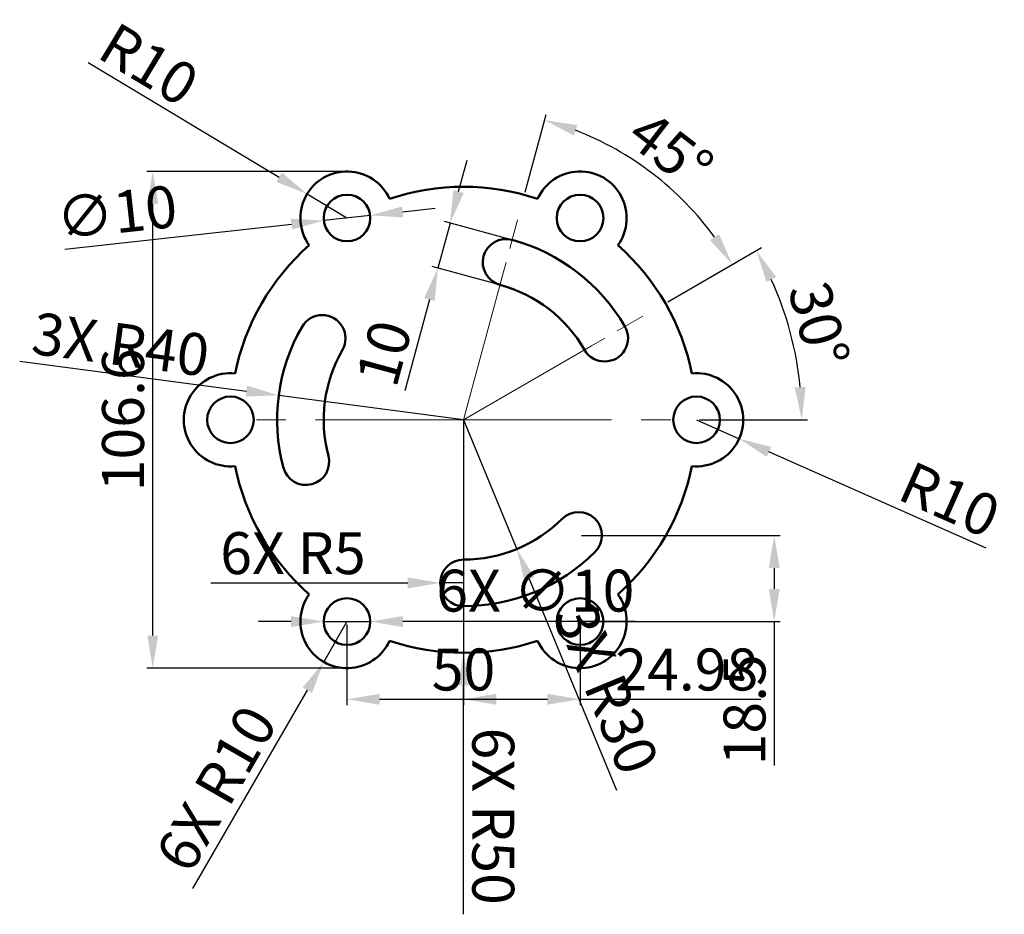
# Model space of a CAD drawing. Units: millimetres. Extents: x 2657 to 2869, y 1596 to 1788.
import ezdxf

# ---------------------------------------------------------------- set-up
doc = ezdxf.new("R2010")
doc.units = ezdxf.units.MM
doc.linetypes.add('CENTER', pattern=[50.8, 31.75, -6.35, 6.35, -6.35])
for name, color, linetype, lineweight in [('M-CNTR', 4, 'CENTER', 18), ('M-CONS', 8, 'Continuous', 13), ('M-DIMS', 2, 'Continuous', 25), ('M-OUTL', 7, 'Continuous', 50)]:
    doc.layers.add(name, color=color, linetype=linetype, lineweight=lineweight)
doc.styles.get("Standard").update_dxf_attribs({"font": 'arial.ttf'})
doc.dimstyles.new('ISO-25', dxfattribs={"dimtxt": 9, "dimasz": 7, "dimexe": 1.25, "dimexo": 0.625, "dimtad": 1, "dimtxsty": 'Standard', "dimcen": 2.5, "dimadec": 0, "dimazin": 0, "dimtfac": 1, "dimtmove": 0, "dimatfit": 3, "dimfxl": 1, "dimarcsym": 0})

# ---------------------------------------------------------------- blocks, each defined once
blk = doc.blocks.new('*D1')
at = {"layer": 'Defpoints', "color": 0, "transparency": 16777216}
for p in [(2765.66, 1750.34), (2799.73, 1749.16), (2795.9, 1727.1), (2752.61, 1702.07), (2752.61, 1702.07)]:
    blk.add_point(p, dxfattribs=at)
at = {"layer": 'M-DIMS', "color": 0, "lineweight": -2, "transparency": 16777216}
for p, q in [((2765.82, 1750.94), (2770.31, 1767.58)), ((2796.44, 1727.41), (2811.36, 1736.04))]:
    blk.add_line(p, q, dxfattribs=at)
blk.add_arc((2752.61, 1702.07), 66.61, 36.0596, 68.8542, dxfattribs=at)
at = {"layer": 'M-DIMS', "color": 0, "transparency": 16777216}
for points in [[(2776.28, 1763.09), (2777, 1765.3), (2769.99, 1766.37)], [(2807.44, 1741.91), (2805.48, 1740.64), (2810.28, 1735.41)]]:
    blk.add_solid(points, dxfattribs=at)
at = {"layer": 'M-DIMS', "color": 0, "transparency": 16777216, "insert": (2796.37, 1759.01), "char_height": 9, "attachment_point": 5, "rotation": 322.4569}
blk.add_mtext('45°', dxfattribs=at)
blk = doc.blocks.new('*D2')
at = {"layer": 'Defpoints', "color": 0, "transparency": 16777216}
for p in [(2795.9, 1727.1), (2824.08, 1714.69), (2752.61, 1702.07), (2752.61, 1702.07), (2802.61, 1702.07)]:
    blk.add_point(p, dxfattribs=at)
at = {"layer": 'M-DIMS', "color": 0, "lineweight": -2, "transparency": 16777216}
for p, q in [((2796.44, 1727.41), (2816.52, 1739.02)), ((2803.24, 1702.07), (2826.44, 1702.07))]:
    blk.add_line(p, q, dxfattribs=at)
blk.add_arc((2752.61, 1702.07), 72.58, 5.5283, 24.5074, dxfattribs=at)
at = {"layer": 'M-DIMS', "color": 0, "transparency": 16777216}
for points in [[(2817.61, 1731.64), (2819.69, 1732.71), (2815.44, 1738.4)], [(2826.02, 1709.12), (2823.69, 1709.01), (2825.19, 1702.07)]]:
    blk.add_solid(points, dxfattribs=at)
at = {"layer": 'M-DIMS', "color": 0, "transparency": 16777216, "insert": (2827.75, 1722.23), "char_height": 9, "attachment_point": 5, "rotation": 285.0179}
blk.add_mtext('30°', dxfattribs=at)
blk = doc.blocks.new('*D3')
at = {"layer": 'Defpoints', "color": 0, "transparency": 16777216}
for p in [(2763.05, 1740.68), (2747.12, 1734.63), (2760.44, 1731.03)]:
    blk.add_point(p, dxfattribs=at)
at = {"layer": 'M-DIMS', "color": 0, "lineweight": -2, "transparency": 16777216}
for p, q in [((2751.55, 1751.04), (2753.38, 1757.8)), ((2749.72, 1744.28), (2747.12, 1734.63)), ((2762.44, 1740.85), (2748.52, 1744.61)), ((2759.83, 1731.19), (2745.91, 1734.96)), ((2745.29, 1727.87), (2740, 1708.31))]:
    blk.add_line(p, q, dxfattribs=at)
at = {"layer": 'M-DIMS', "color": 0, "transparency": 16777216}
for points in [[(2750.42, 1751.35), (2752.68, 1750.74), (2749.72, 1744.28)], [(2744.16, 1728.18), (2746.42, 1727.57), (2747.12, 1734.63)]]:
    blk.add_solid(points, dxfattribs=at)
at = {"layer": 'M-DIMS', "color": 0, "transparency": 16777216, "insert": (2736.69, 1716.08), "char_height": 9, "attachment_point": 5, "rotation": 74.8781}
blk.add_mtext('10', dxfattribs=at)
blk = doc.blocks.new('*D4')
at = {"layer": 'Defpoints', "color": 0, "transparency": 16777216}
for p in [(2719.04, 1750.52), (2727.61, 1745.37)]:
    blk.add_point(p, dxfattribs=at)
at = {"layer": 'M-DIMS', "color": 0, "lineweight": -2, "transparency": 16777216}
for p, q in [((2672.09, 1778.73), (2713.04, 1754.13)), ((2727.61, 1745.37), (2719.04, 1750.52))]:
    blk.add_line(p, q, dxfattribs=at)
at = {"layer": 'M-DIMS', "color": 0, "transparency": 16777216}
blk.add_solid([(2713.64, 1755.13), (2712.44, 1753.13), (2719.04, 1750.52)], dxfattribs=at)
at = {"layer": 'M-DIMS', "color": 0, "transparency": 16777216, "insert": (2684.52, 1777.35), "char_height": 9, "attachment_point": 5, "rotation": 329.0014}
blk.add_mtext('R10', dxfattribs=at)
blk = doc.blocks.new('*D5')
at = {"layer": 'Defpoints', "color": 0, "transparency": 16777216}
for p in [(2802.61, 1702.07), (2811.75, 1698.01)]:
    blk.add_point(p, dxfattribs=at)
at = {"layer": 'M-DIMS', "color": 0, "lineweight": -2, "transparency": 16777216}
for p, q in [((2802.61, 1702.07), (2811.75, 1698.01)), ((2864.72, 1674.51), (2818.15, 1695.18))]:
    blk.add_line(p, q, dxfattribs=at)
at = {"layer": 'M-DIMS', "color": 0, "transparency": 16777216}
blk.add_solid([(2818.62, 1696.24), (2817.68, 1694.11), (2811.75, 1698.01)], dxfattribs=at)
at = {"layer": 'M-DIMS', "color": 0, "transparency": 16777216, "insert": (2856.45, 1683.89), "char_height": 9, "attachment_point": 5, "rotation": 336.0754}
blk.add_mtext('R10', dxfattribs=at)
blk = doc.blocks.new('*D6')
at = {"layer": 'Defpoints', "color": 0, "transparency": 16777216}
for p in [(2732.58, 1745.92), (2722.64, 1744.82)]:
    blk.add_point(p, dxfattribs=at)
at = {"layer": 'M-DIMS', "color": 0, "lineweight": -2, "transparency": 16777216}
for p, q in [((2739.54, 1746.68), (2746.5, 1747.45)), ((2732.58, 1745.92), (2722.64, 1744.82)), ((2667.05, 1738.71), (2715.68, 1744.06))]:
    blk.add_line(p, q, dxfattribs=at)
at = {"layer": 'M-DIMS', "color": 0, "transparency": 16777216}
for points in [[(2739.41, 1747.84), (2739.67, 1745.52), (2732.58, 1745.92)], [(2715.56, 1745.22), (2715.81, 1742.9), (2722.64, 1744.82)]]:
    blk.add_solid(points, dxfattribs=at)
at = {"layer": 'M-DIMS', "color": 0, "transparency": 16777216, "insert": (2678.33, 1745.45), "char_height": 9, "attachment_point": 5, "rotation": 6.2806}
blk.add_mtext('∅10', dxfattribs=at)
blk = doc.blocks.new('MOUNTING-LUG-R10-HOLE-D10')
blk.add_circle((5, 10), 5)
blk.add_arc((5, 10), 10, 264.2608, 95.7392)
blk = doc.blocks.new('ADJUSTMENT-SLOT-R35-W10')
for centre, radius, start, end in [((5, 21.27), 5, 74.8781, 254.8781), ((-4.13, -12.52), 40, 30.0357, 74.8781), ((-4.13, -12.52), 30, 30.0357, 74.8781), ((26.17, 5), 5, 210.0357, 30.0357)]:
    blk.add_arc(centre, radius, start, end)
blk = doc.blocks.new('*D9')
at = {"layer": 'Defpoints', "color": 0, "transparency": 16777216}
for p in [(2685.94, 1755.37), (2727.95, 1755.37), (2727.95, 1648.77)]:
    blk.add_point(p, dxfattribs=at)
at = {"layer": 'M-DIMS', "color": 0, "lineweight": -2, "transparency": 16777216}
for p, q in [((2727.32, 1755.37), (2684.69, 1755.37)), ((2685.94, 1655.77), (2685.94, 1748.37)), ((2727.32, 1648.77), (2684.69, 1648.77))]:
    blk.add_line(p, q, dxfattribs=at)
at = {"layer": 'M-DIMS', "color": 0, "transparency": 16777216}
for points in [[(2684.77, 1748.37), (2687.11, 1748.37), (2685.94, 1755.37)], [(2684.77, 1655.77), (2687.11, 1655.77), (2685.94, 1648.77)]]:
    blk.add_solid(points, dxfattribs=at)
at = {"layer": 'M-DIMS', "color": 0, "transparency": 16777216, "insert": (2680.72, 1702.07), "char_height": 9, "attachment_point": 5, "rotation": 90}
blk.add_mtext('106.6', dxfattribs=at)
blk = doc.blocks.new('*D10')
at = {"layer": 'Defpoints', "color": 0, "transparency": 16777216}
for p in [(2727.61, 1658.77), (2777.61, 1658.77), (2777.61, 1642.1)]:
    blk.add_point(p, dxfattribs=at)
at = {"layer": 'M-DIMS', "color": 0, "lineweight": -2, "transparency": 16777216}
for p, q in [((2727.61, 1658.14), (2727.61, 1640.85)), ((2777.61, 1658.14), (2777.61, 1640.85)), ((2734.61, 1642.1), (2770.61, 1642.1))]:
    blk.add_line(p, q, dxfattribs=at)
at = {"layer": 'M-DIMS', "color": 0, "transparency": 16777216}
for points in [[(2734.61, 1643.27), (2734.61, 1640.94), (2727.61, 1642.1)], [(2770.61, 1643.27), (2770.61, 1640.94), (2777.61, 1642.1)]]:
    blk.add_solid(points, dxfattribs=at)
at = {"layer": 'M-DIMS', "color": 0, "transparency": 16777216, "insert": (2752.61, 1647.32), "char_height": 9, "attachment_point": 5}
blk.add_mtext('50', dxfattribs=at)
blk = doc.blocks.new('*D11')
at = {"layer": 'Defpoints', "color": 0, "transparency": 16777216}
for p in [(2752.63, 1667.07), (2777.61, 1658.77), (2777.61, 1642.1)]:
    blk.add_point(p, dxfattribs=at)
at = {"layer": 'M-DIMS', "color": 0, "lineweight": -2, "transparency": 16777216}
for p, q in [((2752.63, 1666.44), (2752.63, 1640.85)), ((2777.61, 1658.14), (2777.61, 1640.85)), ((2759.63, 1642.1), (2770.61, 1642.1)), ((2777.61, 1642.1), (2816.4, 1642.1))]:
    blk.add_line(p, q, dxfattribs=at)
at = {"layer": 'M-DIMS', "color": 0, "transparency": 16777216}
for points in [[(2759.63, 1643.27), (2759.63, 1640.94), (2752.63, 1642.1)], [(2770.61, 1643.27), (2770.61, 1640.94), (2777.61, 1642.1)]]:
    blk.add_solid(points, dxfattribs=at)
at = {"layer": 'M-DIMS', "color": 0, "transparency": 16777216, "insert": (2800.51, 1647.32), "char_height": 9, "attachment_point": 5}
blk.add_mtext('24.98', dxfattribs=at)
blk = doc.blocks.new('*D12')
at = {"layer": 'Defpoints', "color": 0, "transparency": 16777216}
for p in [(2777.31, 1677.27), (2777.61, 1658.77), (2819.28, 1658.77)]:
    blk.add_point(p, dxfattribs=at)
at = {"layer": 'M-DIMS', "color": 0, "lineweight": -2, "transparency": 16777216}
for p, q in [((2777.93, 1677.27), (2820.53, 1677.27)), ((2819.28, 1670.27), (2819.28, 1665.77)), ((2778.24, 1658.77), (2820.53, 1658.77)), ((2819.28, 1658.77), (2819.28, 1627.92))]:
    blk.add_line(p, q, dxfattribs=at)
at = {"layer": 'M-DIMS', "color": 0, "transparency": 16777216}
for points in [[(2818.11, 1670.27), (2820.45, 1670.27), (2819.28, 1677.27)], [(2818.11, 1665.77), (2820.45, 1665.77), (2819.28, 1658.77)]]:
    blk.add_solid(points, dxfattribs=at)
at = {"layer": 'M-DIMS', "color": 0, "transparency": 16777216, "insert": (2814.06, 1639.84), "char_height": 9, "attachment_point": 5, "rotation": 90}
blk.add_mtext('18.5', dxfattribs=at)
blk = doc.blocks.new('*D13')
at = {"layer": 'Defpoints', "color": 0, "transparency": 16777216}
for p in [(2752.61, 1702.07), (2752.61, 1652.07)]:
    blk.add_point(p, dxfattribs=at)
at = {"layer": 'M-DIMS', "color": 0, "lineweight": -2, "transparency": 16777216}
for p, q in [((2752.61, 1702.07), (2752.61, 1652.07)), ((2752.61, 1595.96), (2752.61, 1645.07))]:
    blk.add_line(p, q, dxfattribs=at)
at = {"layer": 'M-DIMS', "color": 0, "transparency": 16777216}
blk.add_solid([(2753.78, 1645.07), (2751.45, 1645.07), (2752.61, 1652.07)], dxfattribs=at)
at = {"layer": 'M-DIMS', "color": 0, "transparency": 16777216, "insert": (2757.83, 1617.01), "char_height": 9, "attachment_point": 5, "rotation": 270.0005}
blk.add_mtext('6X R50', dxfattribs=at)
blk = doc.blocks.new('*D14')
at = {"layer": 'Defpoints', "color": 0, "transparency": 16777216}
for p in [(2727.61, 1658.77), (2722.61, 1650.11)]:
    blk.add_point(p, dxfattribs=at)
at = {"layer": 'M-DIMS', "color": 0, "lineweight": -2, "transparency": 16777216}
for p, q in [((2727.61, 1658.77), (2722.61, 1650.11)), ((2694.55, 1601.51), (2719.11, 1644.05))]:
    blk.add_line(p, q, dxfattribs=at)
at = {"layer": 'M-DIMS', "color": 0, "transparency": 16777216}
blk.add_solid([(2718.1, 1644.63), (2720.12, 1643.46), (2722.61, 1650.11)], dxfattribs=at)
at = {"layer": 'M-DIMS', "color": 0, "transparency": 16777216, "insert": (2700.56, 1622.36), "char_height": 9, "attachment_point": 5, "rotation": 59.9993}
blk.add_mtext('6X R10', dxfattribs=at)
blk = doc.blocks.new('*D15')
at = {"layer": 'Defpoints', "color": 0, "transparency": 16777216}
for p in [(2722.61, 1658.77), (2732.61, 1658.77)]:
    blk.add_point(p, dxfattribs=at)
at = {"layer": 'M-DIMS', "color": 0, "lineweight": -2, "transparency": 16777216}
for p, q in [((2715.61, 1658.77), (2708.61, 1658.77)), ((2722.61, 1658.77), (2732.61, 1658.77)), ((2789.42, 1658.78), (2739.61, 1658.77))]:
    blk.add_line(p, q, dxfattribs=at)
at = {"layer": 'M-DIMS', "color": 0, "transparency": 16777216}
for points in [[(2715.61, 1659.93), (2715.61, 1657.6), (2722.61, 1658.77)], [(2739.61, 1659.94), (2739.61, 1657.6), (2732.61, 1658.77)]]:
    blk.add_solid(points, dxfattribs=at)
at = {"layer": 'M-DIMS', "color": 0, "transparency": 16777216, "insert": (2768.02, 1664.25), "char_height": 9, "attachment_point": 5, "rotation": 0.0082}
blk.add_mtext('6X ∅10', dxfattribs=at)
blk = doc.blocks.new('*D16')
at = {"layer": 'Defpoints', "color": 0, "transparency": 16777216}
for p in [(2712.96, 1707.32), (2752.61, 1702.07)]:
    blk.add_point(p, dxfattribs=at)
at = {"layer": 'M-DIMS', "color": 0, "lineweight": -2, "transparency": 16777216}
for p, q in [((2657.39, 1714.68), (2706.02, 1708.24)), ((2752.61, 1702.07), (2712.96, 1707.32))]:
    blk.add_line(p, q, dxfattribs=at)
at = {"layer": 'M-DIMS', "color": 0, "transparency": 16777216}
blk.add_solid([(2706.17, 1709.4), (2705.87, 1707.08), (2712.96, 1707.32)], dxfattribs=at)
at = {"layer": 'M-DIMS', "color": 0, "transparency": 16777216, "insert": (2678.92, 1717.1), "char_height": 9, "attachment_point": 5, "rotation": 352.4575}
blk.add_mtext('3X R40', dxfattribs=at)
blk = doc.blocks.new('*D17')
at = {"layer": 'Defpoints', "color": 0, "transparency": 16777216}
for p in [(2752.61, 1702.07), (2764.07, 1674.34)]:
    blk.add_point(p, dxfattribs=at)
at = {"layer": 'M-DIMS', "color": 0, "lineweight": -2, "transparency": 16777216}
for p, q in [((2752.61, 1702.07), (2764.07, 1674.34)), ((2785.48, 1622.54), (2766.75, 1667.88))]:
    blk.add_line(p, q, dxfattribs=at)
at = {"layer": 'M-DIMS', "color": 0, "transparency": 16777216}
blk.add_solid([(2767.82, 1668.32), (2765.67, 1667.43), (2764.07, 1674.34)], dxfattribs=at)
at = {"layer": 'M-DIMS', "color": 0, "transparency": 16777216, "insert": (2782.28, 1643.97), "char_height": 9, "attachment_point": 5, "rotation": 292.4568}
blk.add_mtext('3X R30', dxfattribs=at)
blk = doc.blocks.new('*D18')
at = {"layer": 'Defpoints', "color": 0, "transparency": 16777216}
for p in [(2747.63, 1667.07), (2752.63, 1667.07)]:
    blk.add_point(p, dxfattribs=at)
at = {"layer": 'M-DIMS', "color": 0, "lineweight": -2, "transparency": 16777216}
for p, q in [((2698.42, 1667.07), (2740.63, 1667.07)), ((2752.63, 1667.07), (2747.63, 1667.07))]:
    blk.add_line(p, q, dxfattribs=at)
at = {"layer": 'M-DIMS', "color": 0, "transparency": 16777216}
blk.add_solid([(2740.63, 1668.24), (2740.63, 1665.9), (2747.63, 1667.07)], dxfattribs=at)
at = {"layer": 'M-DIMS', "color": 0, "transparency": 16777216, "insert": (2716.02, 1672.29), "char_height": 9, "attachment_point": 5, "rotation": 359.995}
blk.add_mtext('6X R5', dxfattribs=at)

msp = doc.modelspace()

# ---------------------------------------------------------------- linework, layer by layer
at = {"layer": 'M-CNTR'}
for q in [(2765.655, 1750.338), (2795.897, 1727.097), (2702.612, 1702.07), (2802.612, 1702.07)]:
    msp.add_line((2752.612, 1702.07), q, dxfattribs=at)
at = {"layer": 'M-CONS'}
for p, q in [((2760.438, 1731.031), (2761.742, 1735.858)), ((2778.583, 1717.086), (2782.912, 1719.588))]:
    msp.add_line(p, q, dxfattribs=at)
at = {"layer": 'M-OUTL'}
for start, end in [(71.47834, 108.52166), (131.47834, 168.52166), (11.47834, 48.52166), (191.47834, 228.52166), (311.47834, 348.52166), (251.47834, 288.52166)]:
    msp.add_arc((2752.612, 1702.07), 50, start, end, dxfattribs=at)

# ---------------------------------------------------------------- block references
for name, p, rotation in [('MOUNTING-LUG-R10-HOLE-D10', (2738.771, 1746.041), 120.0000000000249), ('MOUNTING-LUG-R10-HOLE-D10', (2783.772, 1736.041), 60.00000000006959), ('ADJUSTMENT-SLOT-R35-W10', (2739.706, 1699.387), 119.9999999999998), ('MOUNTING-LUG-R10-HOLE-D10', (2707.611, 1712.069), 180), ('ADJUSTMENT-SLOT-R35-W10', (2761.388, 1692.234), 239.9999999999985), ('MOUNTING-LUG-R10-HOLE-D10', (2721.451, 1668.098), 240.00000000001), ('MOUNTING-LUG-R10-HOLE-D10', (2766.452, 1658.098), 300.0000000000274)]:
    msp.add_blockref(name, p, dxfattribs=dict(at, rotation=rotation))
for name, p in [('ADJUSTMENT-SLOT-R35-W10', (2756.741, 1714.588)), ('MOUNTING-LUG-R10-HOLE-D10', (2797.612, 1692.07))]:
    msp.add_blockref(name, p, dxfattribs=at)

# ---------------------------------------------------------------- dimensions: what is measured, and where the dimension line sits
at = {"layer": 'M-DIMS'}
for center, mpoint, picture, middle in [((2727.612, 1745.371), (2719.04, 1750.521), '*D4', (2681.834, 1772.875)), ((2802.612, 1702.07), (2811.752, 1698.014), '*D5', (2854.337, 1679.122))]:
    dim = msp.add_radius_dim(center=center, mpoint=mpoint, dimstyle='ISO-25', override={"dimclrd": 0, "dimclre": 0, "dimclrt": 0}, dxfattribs=at)
    dim.commit()
    dim.dimension.update_dxf_attribs({"geometry": picture, "text_midpoint": middle, "dimtype": 164})
for base, line1, picture, middle in [((2799.726, 1749.156), ((2752.612, 1702.07), (2765.655, 1750.338)), '*D1', (2796.371, 1759.009)), ((2824.083, 1714.687), ((2752.612, 1702.07), (2802.612, 1702.07)), '*D2', (2827.754, 1722.229))]:
    dim = msp.add_angular_dim_2l(base=base, line1=line1, line2=((2752.612, 1702.07), (2795.897, 1727.097)), dimstyle='ISO-25', override={"dimclrd": 0, "dimclre": 0, "dimclrt": 0}, dxfattribs=at)
    dim.commit()
    dim.dimension.update_dxf_attribs({"geometry": picture, "text_midpoint": middle})
dim = msp.add_aligned_dim(p1=(2763.047, 1740.684), p2=(2760.438, 1731.031), distance=-13.801, dimstyle='ISO-25', override={"dimclrd": 0, "dimclre": 0, "dimclrt": 0}, dxfattribs=at)
dim.commit()
dim.dimension.update_dxf_attribs({"geometry": '*D3', "text_midpoint": (2736.693, 1716.075)})
for base, p1, p2, picture, middle in [((2685.942, 1755.365), (2727.945, 1648.774), (2727.945, 1755.365), '*D9', (2680.721, 1702.07)), ((2819.282, 1658.768), (2777.308, 1677.268), (2777.612, 1658.768), '*D12', (2814.061, 1639.844))]:
    dim = msp.add_linear_dim(base=base, p1=p1, p2=p2, angle=90, dimstyle='ISO-25', override={"dimdec": 1, "dimlfac": 1, "dimrnd": 0, "dimzin": 0, "dimdsep": 46, "dimlunit": 2}, dxfattribs=at)
    dim.commit()
    dim.dimension.update_dxf_attribs({"geometry": picture, "text_midpoint": middle})
dim = msp.add_diameter_dim_2p(p1=(2732.582, 1745.918), p2=(2722.642, 1744.824), dimstyle='ISO-25', override={"dimclrd": 0, "dimclre": 0, "dimclrt": 0}, dxfattribs=at)
dim.commit()
dim.dimension.update_dxf_attribs({"geometry": '*D6', "text_midpoint": (2678.932, 1740.013), "dimtype": 163})
for center, mpoint, text, picture, middle in [((2752.612, 1702.07), (2712.958, 1707.32), '3X <>', '*D16', (2678.918, 1717.096)), ((2752.612, 1702.07), (2752.612, 1652.07), '6X <>', '*D13', (2757.832, 1617.013)), ((2752.612, 1702.07), (2764.071, 1674.345), '3X <>', '*D17', (2782.279, 1643.968)), ((2752.633, 1667.07), (2747.633, 1667.07), '6X <>', '*D18', (2716.025, 1672.293)), ((2727.612, 1658.768), (2722.611, 1650.108), '6X <>', '*D14', (2700.562, 1622.359))]:
    dim = msp.add_radius_dim(center=center, mpoint=mpoint, text=text, dimstyle='ISO-25', override={"dimdec": 0, "dimlfac": 1, "dimrnd": 0, "dimzin": 0, "dimdsep": 46, "dimlunit": 2}, dxfattribs=at)
    dim.commit()
    dim.dimension.update_dxf_attribs({"geometry": picture, "text_midpoint": middle})
dim = msp.add_diameter_dim_2p(p1=(2722.612, 1658.768), p2=(2732.612, 1658.769), text='6X <>', dimstyle='ISO-25', override={"dimdec": 0, "dimlfac": 1, "dimrnd": 0, "dimzin": 0, "dimdsep": 46, "dimlunit": 2}, dxfattribs=at)
dim.commit()
dim.dimension.update_dxf_attribs({"geometry": '*D15', "text_midpoint": (2768.018, 1658.774)})
for p1, override, picture, middle in [((2752.633, 1667.07), {"dimdec": 2, "dimlfac": 1, "dimrnd": 0, "dimzin": 0, "dimdsep": 46, "dimlunit": 2}, '*D11', (2800.508, 1647.324)), ((2727.612, 1658.768), {"dimdec": 0, "dimlfac": 1, "dimrnd": 0, "dimzin": 0, "dimdsep": 46, "dimlunit": 2}, '*D10', (2752.612, 1647.324))]:
    dim = msp.add_linear_dim(base=(2777.612, 1642.104), p1=p1, p2=(2777.612, 1658.768), dimstyle='ISO-25', override=override, dxfattribs=at)
    dim.commit()
    dim.dimension.update_dxf_attribs({"geometry": picture, "text_midpoint": middle})

doc.saveas('drawing.dxf')
